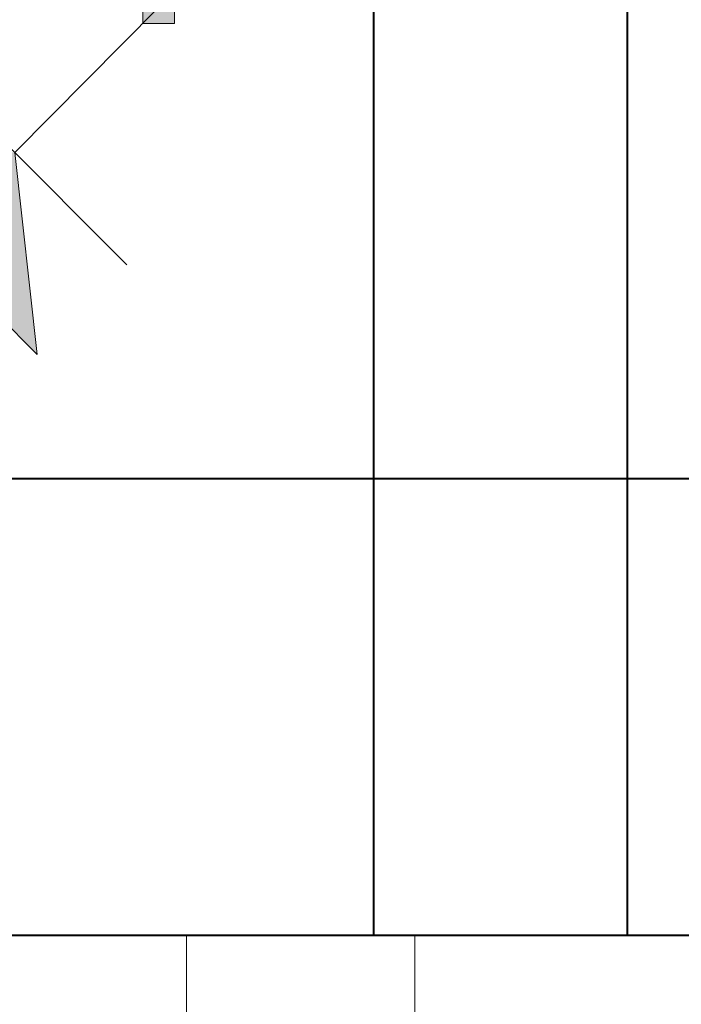
# Model space of a CAD drawing. Units: inches. Extents: x 459864 to 460310, y 324185 to 324787.
# Tile 66 of 112: x 460114.14 to 460127.18, y 324282.12 to 324301.53. Entities that reach past the tile are written whole.
import ezdxf

# ---------------------------------------------------------------- set-up
doc = ezdxf.new("R2010")
doc.units = ezdxf.units.IN
for name, color, linetype, lineweight in [('A-ANNO-DIMS', 2, 'Continuous', 18), ('A-FURN', 8, 'Continuous', 18), ('A-WALL', 7, 'Continuous', 40), ('L-HRDS', 9, 'Continuous', 18), ('L-SITE-PATT', 252, 'Continuous', 13)]:
    doc.layers.add(name, color=color, linetype=linetype, lineweight=lineweight)
doc.styles.get("Standard").update_dxf_attribs({"font": 'arial.ttf'})
doc.dimstyles.new('ISO-25', dxfattribs={"dimtxt": 6, "dimasz": 2.5, "dimexe": 1.25, "dimexo": 0.625, "dimtad": 1, "dimdec": 1, "dimlunit": 3, "dimtxsty": 'Standard', "dimcen": 2.5, "dimadec": 0, "dimazin": 0, "dimtfac": 1, "dimtdec": 1, "dimtmove": 0, "dimatfit": 3, "dimfxl": 1, "dimarcsym": 0})

# ---------------------------------------------------------------- blocks, each defined once
blk = doc.blocks.new('Full Wave Bridge')
for p, q in [((0.486497, -0.114373), (0.6, 0)), ((0.574885, -0.202762), (0.398108, -0.025985)), ((0.504174, -0.273472), (0.327398, -0.096695)), ((0.486497, -0.114373), (0.504174, -0.273472))]:
    blk.add_line(p, q)
blk.add_lwpolyline([(0.5875, -0.0125), (0.5875, 0.0125), (0.6125, 0.0125), (0.6125, -0.0125)], close=True)
for points in [[(0.6125, -0.0125), (0.6125, 0.0125), (0.5875, 0.0125)], [(0.5875, 0.0125), (0.5875, -0.0125), (0.6125, -0.0125)], [(0.327398, -0.096695), (0.486497, -0.114373), (0.504174, -0.273472)]]:
    blk.add_solid(points)
blk = doc.blocks.new('*D28')
at = {"layer": 'A-ANNO-DIMS', "color": 0, "lineweight": -2, "transparency": 16777216}
for p, q in [((460148.65, 324370.7), (460136.025, 324370.7)), ((460137.275, 324368.2), (460137.275, 324293.2)), ((460148.65, 324290.7), (460136.025, 324290.7)), ((460137.275, 324290.7), (460137.275, 324198.69))]:
    blk.add_line(p, q, dxfattribs=at)
at = {"layer": 'A-ANNO-DIMS', "color": 0, "transparency": 16777216}
for points in [[(460136.858, 324368.2), (460137.692, 324368.2), (460137.275, 324370.7)], [(460136.858, 324293.2), (460137.692, 324293.2), (460137.275, 324290.7)]]:
    blk.add_solid(points, dxfattribs=at)
at = {"layer": 'Defpoints', "color": 0, "transparency": 16777216}
for p in [(460149.275, 324370.7), (460137.275, 324290.7), (460149.275, 324290.7)]:
    blk.add_point(p, dxfattribs=at)
at = {"layer": 'A-ANNO-DIMS', "color": 0, "transparency": 16777216, "insert": (460133.363, 324243.445), "char_height": 6, "attachment_point": 5, "rotation": 90}
blk.add_mtext('QUEEN BED 6\'-8" TYP.', dxfattribs=at)

msp = doc.modelspace()

# ---------------------------------------------------------------- hatches: boundary and pattern name
at = {"layer": 'L-SITE-PATT'}
h = msp.add_hatch(dxfattribs=at)
h.set_pattern_fill('DOTS', color=256)
h.paths.add_polyline_path([(460269.804, 324283.483), (460247.115, 324283.483), (460121.929, 324283.483), (460121.929, 324252.473), (460117.429, 324252.473), (460110.124, 324252.473), (460110.124, 324243.287), (460080.83, 324243.287), (460080.83, 324252.473), (460061.115, 324252.473), (460061.115, 324251.882), (460077.909, 324251.882), (460077.909, 324199.483), (460080.83, 324199.483), (460080.83, 324207.553), (460110.124, 324207.553), (460110.124, 324199.483), (460110.813, 324199.483), (460262.115, 324199.483), (460269.804, 324199.483)], flags=17)
edge = h.paths.add_edge_path(flags=0)
edge.add_ellipse((460222.59, 324263.813), major_axis=(-8.485, 8.485), ratio=1, start_angle=405, end_angle=495, ccw=False)
edge.add_line((460214.821, 324254.66), (460214.832, 324254.666))
edge.add_ellipse((460222.59, 324263.813), major_axis=(-8.485, 8.485), ratio=1, start_angle=405, end_angle=495, ccw=False)
edge.add_line((460210.759, 324261.781), (460210.768, 324261.787))
edge.add_ellipse((460222.59, 324263.813), major_axis=(-8.485, 8.485), ratio=1, start_angle=405, end_angle=495, ccw=False)
edge.add_ellipse((460222.59, 324263.813), major_axis=(-8.485, 8.485), ratio=1, start_angle=392.754, end_angle=405, ccw=False)
edge.add_ellipse((460222.59, 324263.813), major_axis=(-8.485, 8.485), ratio=1, start_angle=380.9347, end_angle=392.754, ccw=False)
edge.add_line((460211.337, 324267.985), (460211.34, 324267.985))
edge.add_ellipse((460222.59, 324263.813), major_axis=(-8.485, 8.485), ratio=1, start_angle=380.9347, end_angle=392.754, ccw=False)
edge.add_ellipse((460222.59, 324263.813), major_axis=(-8.485, 8.485), ratio=1, start_angle=347.9015, end_angle=380.9347, ccw=False)
edge.add_ellipse((460222.59, 324263.813), major_axis=(-8.485, 8.485), ratio=1, start_angle=327.0619, end_angle=347.9015, ccw=False)
edge.add_ellipse((460222.59, 324263.813), major_axis=(-8.485, 8.485), ratio=1, start_angle=278.3246, end_angle=327.0619, ccw=False)
edge.add_line((460225.158, 324275.536), (460225.158, 324275.535))
edge.add_ellipse((460222.59, 324263.813), major_axis=(-8.485, 8.485), ratio=1, start_angle=278.3246, end_angle=327.0619, ccw=False)
edge.add_ellipse((460222.59, 324263.813), major_axis=(-8.485, 8.485), ratio=1, start_angle=260.6436, end_angle=278.3246, ccw=False)
edge.add_ellipse((460222.59, 324263.813), major_axis=(-8.485, 8.485), ratio=1, start_angle=225, end_angle=260.6436, ccw=False)
edge.add_line((460234.509, 324265.243), (460234.501, 324265.239))
edge.add_ellipse((460222.59, 324263.813), major_axis=(-8.485, 8.485), ratio=1, start_angle=225, end_angle=260.6436, ccw=False)
edge.add_ellipse((460222.59, 324263.813), major_axis=(-8.485, 8.485), ratio=1, start_angle=495, end_angle=585, ccw=False)
edge.add_line((460234.437, 324261.861), (460234.424, 324261.858))
edge.add_ellipse((460222.59, 324263.813), major_axis=(-8.485, 8.485), ratio=1, start_angle=495, end_angle=585, ccw=False)
edge.add_line((460227.95, 324253.067), (460227.946, 324253.083))
edge.add_ellipse((460222.59, 324263.813), major_axis=(-8.485, 8.485), ratio=1, start_angle=495, end_angle=585, ccw=False)
edge.add_line((460226.223, 324252.369), (460226.211, 324252.38))
edge.add_ellipse((460222.59, 324263.813), major_axis=(-8.485, 8.485), ratio=1, start_angle=495, end_angle=585, ccw=False)
h.paths.add_polyline_path([(460219.651, 324254.347), (460218.461, 324253.545), (460218.275, 324254.789), (460219.642, 324256.542), (460219.625, 324260.848), (460216.11, 324257.333), (460214.35, 324256.978), (460215.416, 324259.356), (460212.524, 324258.496), (460213.137, 324259.93), (460218.507, 324263.813), (460222.59, 324263.813), (460222.59, 324267.807), (460218.176, 324272.212), (460219.026, 324274.639), (460222.59, 324272.811), (460222.59, 324275.423), (460223.057, 324274.825), (460222.675, 324273.492), (460225.912, 324267.135), (460219.625, 324260.848)], flags=0)
edge = h.paths.add_edge_path(flags=0)
edge.add_ellipse((460194.576, 324264.046), major_axis=(-8.485, 8.485), ratio=1, start_angle=495, end_angle=585, ccw=False)
edge.add_line((460199.936, 324253.3), (460199.932, 324253.316))
edge.add_ellipse((460194.576, 324264.046), major_axis=(-8.485, 8.485), ratio=1, start_angle=495, end_angle=585, ccw=False)
edge.add_line((460198.208, 324252.603), (460198.196, 324252.613))
edge.add_ellipse((460194.576, 324264.046), major_axis=(-8.485, 8.485), ratio=1, start_angle=495, end_angle=585, ccw=False)
edge.add_ellipse((460194.576, 324264.046), major_axis=(-8.485, 8.485), ratio=1, start_angle=405, end_angle=495, ccw=False)
edge.add_line((460186.806, 324254.893), (460186.817, 324254.899))
edge.add_ellipse((460194.576, 324264.046), major_axis=(-8.485, 8.485), ratio=1, start_angle=405, end_angle=495, ccw=False)
edge.add_line((460182.744, 324262.014), (460182.753, 324262.02))
edge.add_ellipse((460194.576, 324264.046), major_axis=(-8.485, 8.485), ratio=1, start_angle=405, end_angle=495, ccw=False)
edge.add_ellipse((460194.576, 324264.046), major_axis=(-8.485, 8.485), ratio=1, start_angle=392.754, end_angle=405, ccw=False)
edge.add_ellipse((460194.576, 324264.046), major_axis=(-8.485, 8.485), ratio=1, start_angle=380.9347, end_angle=392.754, ccw=False)
edge.add_line((460183.323, 324268.218), (460183.326, 324268.218))
edge.add_ellipse((460194.576, 324264.046), major_axis=(-8.485, 8.485), ratio=1, start_angle=380.9347, end_angle=392.754, ccw=False)
edge.add_ellipse((460194.576, 324264.046), major_axis=(-8.485, 8.485), ratio=1, start_angle=347.9015, end_angle=380.9347, ccw=False)
edge.add_ellipse((460194.576, 324264.046), major_axis=(-8.485, 8.485), ratio=1, start_angle=327.0619, end_angle=347.9015, ccw=False)
edge.add_ellipse((460194.576, 324264.046), major_axis=(-8.485, 8.485), ratio=1, start_angle=278.3246, end_angle=327.0619, ccw=False)
edge.add_line((460197.144, 324275.769), (460197.143, 324275.768))
edge.add_ellipse((460194.576, 324264.046), major_axis=(-8.485, 8.485), ratio=1, start_angle=278.3246, end_angle=327.0619, ccw=False)
edge.add_ellipse((460194.576, 324264.046), major_axis=(-8.485, 8.485), ratio=1, start_angle=260.6436, end_angle=278.3246, ccw=False)
edge.add_ellipse((460194.576, 324264.046), major_axis=(-8.485, 8.485), ratio=1, start_angle=225, end_angle=260.6436, ccw=False)
edge.add_line((460206.494, 324265.476), (460206.487, 324265.473))
edge.add_ellipse((460194.576, 324264.046), major_axis=(-8.485, 8.485), ratio=1, start_angle=225, end_angle=260.6436, ccw=False)
edge.add_ellipse((460194.576, 324264.046), major_axis=(-8.485, 8.485), ratio=1, start_angle=495, end_angle=585, ccw=False)
edge.add_line((460206.422, 324262.094), (460206.409, 324262.091))
h.paths.add_polyline_path([(460191.61, 324261.081), (460191.637, 324254.58), (460190.447, 324253.778), (460190.261, 324255.023), (460191.628, 324256.775), (460191.61, 324261.081), (460188.096, 324257.566), (460186.335, 324257.211), (460187.402, 324259.589), (460184.509, 324258.729), (460185.123, 324260.163), (460190.493, 324264.046), (460194.576, 324264.046), (460194.576, 324268.04), (460190.161, 324272.446), (460191.011, 324274.872), (460194.576, 324273.044), (460194.576, 324275.657), (460195.043, 324275.058), (460194.661, 324273.725), (460197.897, 324267.368)], flags=0)
edge = h.paths.add_edge_path(flags=0)
edge.add_ellipse((460252.912, 324263.578), major_axis=(-8.485, 8.485), ratio=1, start_angle=405, end_angle=495, ccw=False)
edge.add_line((460241.081, 324261.545), (460241.089, 324261.551))
edge.add_ellipse((460252.912, 324263.578), major_axis=(-8.485, 8.485), ratio=1, start_angle=405, end_angle=495, ccw=False)
edge.add_ellipse((460252.912, 324263.578), major_axis=(-8.485, 8.485), ratio=1, start_angle=392.754, end_angle=405, ccw=False)
edge.add_ellipse((460252.912, 324263.578), major_axis=(-8.485, 8.485), ratio=1, start_angle=380.9347, end_angle=392.754, ccw=False)
edge.add_line((460241.659, 324267.749), (460241.662, 324267.749))
edge.add_ellipse((460252.912, 324263.578), major_axis=(-8.485, 8.485), ratio=1, start_angle=380.9347, end_angle=392.754, ccw=False)
edge.add_ellipse((460252.912, 324263.578), major_axis=(-8.485, 8.485), ratio=1, start_angle=347.9015, end_angle=380.9347, ccw=False)
edge.add_ellipse((460252.912, 324263.578), major_axis=(-8.485, 8.485), ratio=1, start_angle=327.0619, end_angle=347.9015, ccw=False)
edge.add_ellipse((460252.912, 324263.578), major_axis=(-8.485, 8.485), ratio=1, start_angle=278.3246, end_angle=327.0619, ccw=False)
edge.add_line((460255.48, 324275.3), (460255.479, 324275.299))
edge.add_ellipse((460252.912, 324263.578), major_axis=(-8.485, 8.485), ratio=1, start_angle=278.3246, end_angle=327.0619, ccw=False)
edge.add_ellipse((460252.912, 324263.578), major_axis=(-8.485, 8.485), ratio=1, start_angle=260.6436, end_angle=278.3246, ccw=False)
edge.add_ellipse((460252.912, 324263.578), major_axis=(-8.485, 8.485), ratio=1, start_angle=225, end_angle=260.6436, ccw=False)
edge.add_line((460264.83, 324265.007), (460264.823, 324265.004))
edge.add_ellipse((460252.912, 324263.578), major_axis=(-8.485, 8.485), ratio=1, start_angle=225, end_angle=260.6436, ccw=False)
edge.add_ellipse((460252.912, 324263.578), major_axis=(-8.485, 8.485), ratio=1, start_angle=495, end_angle=585, ccw=False)
edge.add_line((460264.758, 324261.626), (460264.745, 324261.622))
edge.add_ellipse((460252.912, 324263.578), major_axis=(-8.485, 8.485), ratio=1, start_angle=495, end_angle=585, ccw=False)
edge.add_line((460258.272, 324252.832), (460258.268, 324252.848))
edge.add_ellipse((460252.912, 324263.578), major_axis=(-8.485, 8.485), ratio=1, start_angle=495, end_angle=585, ccw=False)
edge.add_line((460256.545, 324252.134), (460256.533, 324252.144))
edge.add_ellipse((460252.912, 324263.578), major_axis=(-8.485, 8.485), ratio=1, start_angle=495, end_angle=585, ccw=False)
edge.add_ellipse((460252.912, 324263.578), major_axis=(-8.485, 8.485), ratio=1, start_angle=405, end_angle=495, ccw=False)
edge.add_line((460245.143, 324254.424), (460245.153, 324254.43))
h.paths.add_polyline_path([(460244.672, 324256.742), (460245.738, 324259.12), (460242.846, 324258.26), (460243.459, 324259.694), (460248.829, 324263.578), (460252.912, 324263.578), (460252.912, 324267.571), (460248.497, 324271.977), (460249.348, 324274.403), (460252.912, 324272.576), (460252.912, 324275.188), (460253.379, 324274.589), (460252.997, 324273.257), (460256.233, 324266.899), (460249.946, 324260.612), (460249.973, 324254.111), (460248.783, 324253.309), (460248.597, 324254.554), (460249.964, 324256.306), (460249.946, 324260.612), (460246.432, 324257.097)], flags=0)
edge = h.paths.add_edge_path(flags=0)
edge.add_ellipse((460167.439, 324262.833), major_axis=(-8.485, 8.485), ratio=1, start_angle=495, end_angle=585, ccw=False)
edge.add_line((460172.799, 324252.087), (460172.795, 324252.103))
edge.add_ellipse((460167.439, 324262.833), major_axis=(-8.485, 8.485), ratio=1, start_angle=495, end_angle=585, ccw=False)
edge.add_line((460171.071, 324251.389), (460171.059, 324251.399))
edge.add_ellipse((460167.439, 324262.833), major_axis=(-8.485, 8.485), ratio=1, start_angle=495, end_angle=585, ccw=False)
edge.add_ellipse((460167.439, 324262.833), major_axis=(-8.485, 8.485), ratio=1, start_angle=405, end_angle=495, ccw=False)
edge.add_line((460159.669, 324253.679), (460159.68, 324253.685))
edge.add_ellipse((460167.439, 324262.833), major_axis=(-8.485, 8.485), ratio=1, start_angle=405, end_angle=495, ccw=False)
edge.add_line((460155.607, 324260.8), (460155.616, 324260.806))
edge.add_ellipse((460167.439, 324262.833), major_axis=(-8.485, 8.485), ratio=1, start_angle=405, end_angle=495, ccw=False)
edge.add_ellipse((460167.439, 324262.833), major_axis=(-8.485, 8.485), ratio=1, start_angle=392.754, end_angle=405, ccw=False)
edge.add_ellipse((460167.439, 324262.833), major_axis=(-8.485, 8.485), ratio=1, start_angle=380.9347, end_angle=392.754, ccw=False)
edge.add_line((460156.185, 324267.005), (460156.189, 324267.005))
edge.add_ellipse((460167.439, 324262.833), major_axis=(-8.485, 8.485), ratio=1, start_angle=380.9347, end_angle=392.754, ccw=False)
edge.add_ellipse((460167.439, 324262.833), major_axis=(-8.485, 8.485), ratio=1, start_angle=347.9015, end_angle=380.9347, ccw=False)
edge.add_ellipse((460167.439, 324262.833), major_axis=(-8.485, 8.485), ratio=1, start_angle=327.0619, end_angle=347.9015, ccw=False)
edge.add_ellipse((460167.439, 324262.833), major_axis=(-8.485, 8.485), ratio=1, start_angle=278.3246, end_angle=327.0619, ccw=False)
edge.add_line((460170.007, 324274.556), (460170.006, 324274.554))
edge.add_ellipse((460167.439, 324262.833), major_axis=(-8.485, 8.485), ratio=1, start_angle=278.3246, end_angle=327.0619, ccw=False)
edge.add_ellipse((460167.439, 324262.833), major_axis=(-8.485, 8.485), ratio=1, start_angle=260.6436, end_angle=278.3246, ccw=False)
edge.add_ellipse((460167.439, 324262.833), major_axis=(-8.485, 8.485), ratio=1, start_angle=225, end_angle=260.6436, ccw=False)
edge.add_line((460179.357, 324264.262), (460179.35, 324264.259))
edge.add_ellipse((460167.439, 324262.833), major_axis=(-8.485, 8.485), ratio=1, start_angle=225, end_angle=260.6436, ccw=False)
edge.add_ellipse((460167.439, 324262.833), major_axis=(-8.485, 8.485), ratio=1, start_angle=495, end_angle=585, ccw=False)
edge.add_line((460179.285, 324260.881), (460179.272, 324260.877))
h.paths.add_polyline_path([(460164.473, 324259.867), (460164.5, 324253.366), (460163.31, 324252.565), (460163.124, 324253.809), (460164.491, 324255.561), (460164.473, 324259.867), (460160.958, 324256.353), (460159.198, 324255.998), (460160.265, 324258.375), (460157.372, 324257.515), (460157.986, 324258.949), (460163.356, 324262.833), (460167.439, 324262.833), (460167.439, 324266.826), (460163.024, 324271.232), (460163.874, 324273.659), (460167.439, 324271.831), (460167.439, 324274.443), (460167.905, 324273.844), (460167.524, 324272.512), (460170.76, 324266.154)], flags=0)
edge = h.paths.add_edge_path(flags=0)
edge.add_ellipse((460140.758, 324262.37), major_axis=(-8.485, 8.485), ratio=1, start_angle=495, end_angle=585, ccw=False)
edge.add_line((460146.118, 324251.624), (460146.114, 324251.639))
edge.add_ellipse((460140.758, 324262.37), major_axis=(-8.485, 8.485), ratio=1, start_angle=495, end_angle=585, ccw=False)
edge.add_line((460144.391, 324250.926), (460144.379, 324250.936))
edge.add_ellipse((460140.758, 324262.37), major_axis=(-8.485, 8.485), ratio=1, start_angle=495, end_angle=585, ccw=False)
edge.add_ellipse((460140.758, 324262.37), major_axis=(-8.485, 8.485), ratio=1, start_angle=405, end_angle=495, ccw=False)
edge.add_line((460132.989, 324253.216), (460132.999, 324253.222))
edge.add_ellipse((460140.758, 324262.37), major_axis=(-8.485, 8.485), ratio=1, start_angle=405, end_angle=495, ccw=False)
edge.add_line((460128.927, 324260.337), (460128.935, 324260.343))
edge.add_ellipse((460140.758, 324262.37), major_axis=(-8.485, 8.485), ratio=1, start_angle=405, end_angle=495, ccw=False)
edge.add_ellipse((460140.758, 324262.37), major_axis=(-8.485, 8.485), ratio=1, start_angle=392.754, end_angle=405, ccw=False)
edge.add_ellipse((460140.758, 324262.37), major_axis=(-8.485, 8.485), ratio=1, start_angle=380.9347, end_angle=392.754, ccw=False)
edge.add_line((460129.505, 324266.541), (460129.508, 324266.541))
edge.add_ellipse((460140.758, 324262.37), major_axis=(-8.485, 8.485), ratio=1, start_angle=380.9347, end_angle=392.754, ccw=False)
edge.add_ellipse((460140.758, 324262.37), major_axis=(-8.485, 8.485), ratio=1, start_angle=347.9015, end_angle=380.9347, ccw=False)
edge.add_ellipse((460140.758, 324262.37), major_axis=(-8.485, 8.485), ratio=1, start_angle=327.0619, end_angle=347.9015, ccw=False)
edge.add_ellipse((460140.758, 324262.37), major_axis=(-8.485, 8.485), ratio=1, start_angle=278.3246, end_angle=327.0619, ccw=False)
edge.add_line((460143.326, 324274.092), (460143.325, 324274.091))
edge.add_ellipse((460140.758, 324262.37), major_axis=(-8.485, 8.485), ratio=1, start_angle=278.3246, end_angle=327.0619, ccw=False)
edge.add_ellipse((460140.758, 324262.37), major_axis=(-8.485, 8.485), ratio=1, start_angle=260.6436, end_angle=278.3246, ccw=False)
edge.add_ellipse((460140.758, 324262.37), major_axis=(-8.485, 8.485), ratio=1, start_angle=225, end_angle=260.6436, ccw=False)
edge.add_line((460152.677, 324263.799), (460152.669, 324263.796))
edge.add_ellipse((460140.758, 324262.37), major_axis=(-8.485, 8.485), ratio=1, start_angle=225, end_angle=260.6436, ccw=False)
edge.add_ellipse((460140.758, 324262.37), major_axis=(-8.485, 8.485), ratio=1, start_angle=495, end_angle=585, ccw=False)
edge.add_line((460152.604, 324260.418), (460152.592, 324260.414))
h.paths.add_polyline_path([(460137.792, 324259.404), (460137.819, 324252.903), (460136.629, 324252.101), (460136.443, 324253.346), (460137.81, 324255.098), (460137.792, 324259.404), (460134.278, 324255.889), (460132.518, 324255.534), (460133.584, 324257.912), (460130.692, 324257.052), (460131.305, 324258.486), (460136.675, 324262.37), (460140.758, 324262.37), (460140.758, 324266.363), (460136.343, 324270.769), (460137.194, 324273.195), (460140.758, 324271.367), (460140.758, 324273.98), (460141.225, 324273.381), (460140.843, 324272.049), (460144.079, 324265.691)], flags=0)
h.paths.add_polyline_path([(460110.124, 324227.414), (460080.83, 324227.414), (460080.83, 324235.484), (460110.124, 324235.484)], flags=16)
h.paths.add_polyline_path([(460110.124, 324220.797), (460110.124, 324212.727), (460080.83, 324212.727), (460080.83, 324220.797)], flags=16)
h.paths.add_polyline_path([(460269.804, 324283.483), (460247.115, 324283.483), (460121.929, 324283.483), (460121.929, 324252.473), (460117.429, 324252.473), (460110.124, 324252.473), (460110.124, 324243.287), (460080.83, 324243.287), (460080.83, 324252.473), (460061.115, 324252.473), (460061.115, 324251.882), (460077.909, 324251.882), (460077.909, 324199.483), (460080.83, 324199.483), (460080.83, 324207.553), (460110.124, 324207.553), (460110.124, 324199.483), (460262.115, 324199.483), (460269.804, 324199.483)], flags=17)
h.paths.add_polyline_path([(460219.651, 324254.347), (460218.461, 324253.545), (460218.275, 324254.789), (460219.642, 324256.542), (460219.625, 324260.848), (460216.11, 324257.333), (460214.35, 324256.978), (460215.416, 324259.356), (460212.524, 324258.496), (460213.137, 324259.93), (460218.507, 324263.813), (460222.59, 324263.813), (460220.18, 324266.223), (460215.461, 324265.308), (460211.835, 324266.137), (460216.247, 324267.985), (460218.418, 324267.985), (460222.59, 324263.813), (460222.59, 324267.807), (460218.176, 324272.212), (460219.026, 324274.639), (460222.59, 324272.811), (460222.59, 324275.423), (460223.057, 324274.825), (460222.675, 324273.492), (460225.912, 324267.135), (460222.59, 324263.813), (460231.383, 324263.813), (460228.485, 324262.488), (460224.425, 324261.978), (460228.68, 324257.724), (460228.966, 324254.791), (460227.142, 324256.537), (460227.542, 324254.819), (460227.333, 324253.614), (460222.59, 324259.985), (460222.59, 324255.497), (460221.377, 324256.541), (460220.576, 324261.799), (460219.625, 324260.848)], flags=0)
h.paths.add_polyline_path([(460199.127, 324256.77), (460199.528, 324255.052), (460199.319, 324253.848), (460194.576, 324260.218), (460194.576, 324255.73), (460193.363, 324256.774), (460192.561, 324262.032), (460191.61, 324261.081), (460191.637, 324254.58), (460190.447, 324253.778), (460190.261, 324255.023), (460191.628, 324256.775), (460191.61, 324261.081), (460188.096, 324257.566), (460186.335, 324257.211), (460187.402, 324259.589), (460184.509, 324258.729), (460185.123, 324260.163), (460190.493, 324264.046), (460194.576, 324264.046), (460192.166, 324266.456), (460187.446, 324265.541), (460183.82, 324266.37), (460188.232, 324268.218), (460190.404, 324268.218), (460194.576, 324264.046), (460194.576, 324268.04), (460190.161, 324272.446), (460191.011, 324274.872), (460194.576, 324273.044), (460194.576, 324275.657), (460195.043, 324275.058), (460194.661, 324273.725), (460197.897, 324267.368), (460194.576, 324264.046), (460203.368, 324264.046), (460200.47, 324262.721), (460196.411, 324262.212), (460200.665, 324257.957), (460200.951, 324255.024)], flags=0)
h.paths.add_polyline_path([(460244.672, 324256.742), (460245.738, 324259.12), (460242.846, 324258.26), (460243.459, 324259.694), (460248.829, 324263.578), (460252.912, 324263.578), (460250.502, 324265.987), (460245.783, 324265.072), (460242.156, 324265.901), (460246.568, 324267.749), (460248.74, 324267.749), (460252.912, 324263.578), (460252.912, 324267.571), (460248.497, 324271.977), (460249.348, 324274.403), (460252.912, 324272.576), (460252.912, 324275.188), (460253.379, 324274.589), (460252.997, 324273.257), (460256.233, 324266.899), (460252.912, 324263.578), (460261.705, 324263.578), (460258.806, 324262.252), (460254.747, 324261.743), (460259.002, 324257.488), (460259.288, 324254.555), (460257.463, 324256.301), (460257.864, 324254.583), (460257.655, 324253.379), (460252.912, 324259.749), (460252.912, 324255.261), (460251.699, 324256.305), (460250.897, 324261.563), (460249.946, 324260.612), (460249.973, 324254.111), (460248.783, 324253.309), (460248.597, 324254.554), (460249.964, 324256.306), (460249.946, 324260.612), (460246.432, 324257.097)], flags=0)
h.paths.add_polyline_path([(460173.528, 324256.743), (460173.814, 324253.811), (460171.99, 324255.556), (460172.39, 324253.838), (460172.182, 324252.634), (460167.439, 324259.004), (460167.439, 324254.516), (460166.226, 324255.56), (460165.424, 324260.818), (460164.473, 324259.867), (460164.5, 324253.366), (460163.31, 324252.565), (460163.124, 324253.809), (460164.491, 324255.561), (460164.473, 324259.867), (460160.958, 324256.353), (460159.198, 324255.998), (460160.265, 324258.375), (460157.372, 324257.515), (460157.986, 324258.949), (460163.356, 324262.833), (460167.439, 324262.833), (460165.029, 324265.243), (460160.309, 324264.327), (460156.683, 324265.156), (460161.095, 324267.005), (460163.267, 324267.005), (460167.439, 324262.833), (460167.439, 324266.826), (460163.024, 324271.232), (460163.874, 324273.659), (460167.439, 324271.831), (460167.439, 324274.443), (460167.905, 324273.844), (460167.524, 324272.512), (460170.76, 324266.154), (460167.439, 324262.833), (460176.231, 324262.833), (460173.333, 324261.507), (460169.274, 324260.998)], flags=0)
h.paths.add_polyline_path([(460146.848, 324256.28), (460147.134, 324253.347), (460145.31, 324255.093), (460145.71, 324253.375), (460145.501, 324252.171), (460140.758, 324258.541), (460140.758, 324254.053), (460139.545, 324255.097), (460138.744, 324260.355), (460137.792, 324259.404), (460137.819, 324252.903), (460136.629, 324252.101), (460136.443, 324253.346), (460137.81, 324255.098), (460137.792, 324259.404), (460134.278, 324255.889), (460132.518, 324255.534), (460133.584, 324257.912), (460130.692, 324257.052), (460131.305, 324258.486), (460136.675, 324262.37), (460140.758, 324262.37), (460138.348, 324264.779), (460133.629, 324263.864), (460130.002, 324264.693), (460134.414, 324266.541), (460136.586, 324266.541), (460140.758, 324262.37), (460140.758, 324266.363), (460136.343, 324270.769), (460137.194, 324273.195), (460140.758, 324271.367), (460140.758, 324273.98), (460141.225, 324273.381), (460140.843, 324272.049), (460144.079, 324265.691), (460140.758, 324262.37), (460149.551, 324262.37), (460146.653, 324261.044), (460142.593, 324260.535)], flags=0)
edge = h.paths.add_edge_path()
edge.add_line((460269.804, 324272.549), (460260.881, 324272.549))
edge.add_ellipse((460252.912, 324263.578), major_axis=(-8.485, 8.485), ratio=1, start_angle=260.6436, end_angle=273.3846, ccw=False)
edge.add_line((460262.283, 324271.092), (460262.261, 324271.091))
edge.add_ellipse((460252.912, 324263.578), major_axis=(-8.485, 8.485), ratio=1, start_angle=260.6436, end_angle=273.3846, ccw=False)
edge.add_ellipse((460252.912, 324263.578), major_axis=(-8.485, 8.485), ratio=1, start_angle=225, end_angle=260.6436, ccw=False)
edge.add_line((460263.609, 324269.063), (460263.572, 324269.058))
edge.add_ellipse((460252.912, 324263.578), major_axis=(-8.485, 8.485), ratio=1, start_angle=225, end_angle=260.6436, ccw=False)
edge.add_line((460264.615, 324266.306), (460264.585, 324266.305))
edge.add_ellipse((460252.912, 324263.578), major_axis=(-8.485, 8.485), ratio=1, start_angle=225, end_angle=260.6436, ccw=False)
edge.add_line((460264.83, 324265.007), (460264.823, 324265.004))
edge.add_ellipse((460252.912, 324263.578), major_axis=(-8.485, 8.485), ratio=1, start_angle=225, end_angle=260.6436, ccw=False)
edge.add_ellipse((460252.912, 324263.578), major_axis=(-8.485, 8.485), ratio=1, start_angle=495, end_angle=585, ccw=False)
edge.add_line((460264.758, 324261.626), (460264.745, 324261.622))
edge.add_ellipse((460252.912, 324263.578), major_axis=(-8.485, 8.485), ratio=1, start_angle=495, end_angle=585, ccw=False)
edge.add_line((460263.442, 324257.739), (460263.389, 324257.779))
edge.add_ellipse((460252.912, 324263.578), major_axis=(-8.485, 8.485), ratio=1, start_angle=495, end_angle=585, ccw=False)
edge.add_line((460258.128, 324252.744), (460258.102, 324252.779))
edge.add_ellipse((460252.912, 324263.578), major_axis=(-8.485, 8.485), ratio=1, start_angle=495, end_angle=585, ccw=False)
edge.add_line((460256.545, 324252.134), (460256.533, 324252.144))
edge.add_ellipse((460252.912, 324263.578), major_axis=(-8.485, 8.485), ratio=1, start_angle=495, end_angle=585, ccw=False)
edge.add_ellipse((460252.912, 324263.578), major_axis=(-8.485, 8.485), ratio=1, start_angle=405, end_angle=495, ccw=False)
edge.add_line((460250.594, 324251.78), (460250.605, 324251.82))
edge.add_ellipse((460252.912, 324263.578), major_axis=(-8.485, 8.485), ratio=1, start_angle=405, end_angle=495, ccw=False)
edge.add_line((460245.143, 324254.424), (460245.153, 324254.43))
edge.add_ellipse((460252.912, 324263.578), major_axis=(-8.485, 8.485), ratio=1, start_angle=405, end_angle=495, ccw=False)
edge.add_line((460243.525, 324256.059), (460243.56, 324256.091))
edge.add_ellipse((460252.912, 324263.578), major_axis=(-8.485, 8.485), ratio=1, start_angle=405, end_angle=495, ccw=False)
edge.add_line((460241.44, 324259.893), (460241.522, 324259.896))
edge.add_ellipse((460252.912, 324263.578), major_axis=(-8.485, 8.485), ratio=1, start_angle=405, end_angle=495, ccw=False)
edge.add_line((460241.081, 324261.545), (460241.089, 324261.551))
edge.add_ellipse((460252.912, 324263.578), major_axis=(-8.485, 8.485), ratio=1, start_angle=405, end_angle=495, ccw=False)
edge.add_ellipse((460252.912, 324263.578), major_axis=(-8.485, 8.485), ratio=1, start_angle=392.754, end_angle=405, ccw=False)
edge.add_line((460241.05, 324265.438), (460241.063, 324265.443))
edge.add_ellipse((460252.912, 324263.578), major_axis=(-8.485, 8.485), ratio=1, start_angle=392.754, end_angle=405, ccw=False)
edge.add_ellipse((460252.912, 324263.578), major_axis=(-8.485, 8.485), ratio=1, start_angle=380.9347, end_angle=392.754, ccw=False)
edge.add_line((460241.452, 324267.176), (460241.469, 324267.171))
edge.add_ellipse((460252.912, 324263.578), major_axis=(-8.485, 8.485), ratio=1, start_angle=380.9347, end_angle=392.754, ccw=False)
edge.add_line((460241.659, 324267.749), (460241.662, 324267.749))
edge.add_ellipse((460252.912, 324263.578), major_axis=(-8.485, 8.485), ratio=1, start_angle=380.9347, end_angle=392.754, ccw=False)
edge.add_ellipse((460252.912, 324263.578), major_axis=(-8.485, 8.485), ratio=1, start_angle=356.6154, end_angle=380.9347, ccw=False)
edge.add_line((460244.88, 324272.488), (460244.713, 324272.549))
edge.add_line((460244.713, 324272.549), (460230.817, 324272.549))
edge.add_ellipse((460222.59, 324263.813), major_axis=(-8.485, 8.485), ratio=1, start_angle=260.6436, end_angle=271.7178, ccw=False)
edge.add_ellipse((460222.59, 324263.813), major_axis=(-8.485, 8.485), ratio=1, start_angle=225, end_angle=260.6436, ccw=False)
edge.add_line((460233.287, 324269.299), (460233.25, 324269.294))
edge.add_ellipse((460222.59, 324263.813), major_axis=(-8.485, 8.485), ratio=1, start_angle=225, end_angle=260.6436, ccw=False)
edge.add_line((460234.294, 324266.541), (460234.264, 324266.541))
edge.add_ellipse((460222.59, 324263.813), major_axis=(-8.485, 8.485), ratio=1, start_angle=225, end_angle=260.6436, ccw=False)
edge.add_line((460234.509, 324265.243), (460234.501, 324265.239))
edge.add_ellipse((460222.59, 324263.813), major_axis=(-8.485, 8.485), ratio=1, start_angle=225, end_angle=260.6436, ccw=False)
edge.add_ellipse((460222.59, 324263.813), major_axis=(-8.485, 8.485), ratio=1, start_angle=495, end_angle=585, ccw=False)
edge.add_line((460234.437, 324261.861), (460234.424, 324261.858))
edge.add_ellipse((460222.59, 324263.813), major_axis=(-8.485, 8.485), ratio=1, start_angle=495, end_angle=585, ccw=False)
edge.add_line((460233.121, 324257.975), (460233.068, 324258.015))
edge.add_ellipse((460222.59, 324263.813), major_axis=(-8.485, 8.485), ratio=1, start_angle=495, end_angle=585, ccw=False)
edge.add_line((460227.806, 324252.979), (460227.78, 324253.014))
edge.add_ellipse((460222.59, 324263.813), major_axis=(-8.485, 8.485), ratio=1, start_angle=495, end_angle=585, ccw=False)
edge.add_line((460226.223, 324252.369), (460226.211, 324252.38))
edge.add_ellipse((460222.59, 324263.813), major_axis=(-8.485, 8.485), ratio=1, start_angle=495, end_angle=585, ccw=False)
edge.add_ellipse((460222.59, 324263.813), major_axis=(-8.485, 8.485), ratio=1, start_angle=405, end_angle=495, ccw=False)
edge.add_line((460220.272, 324252.016), (460220.283, 324252.055))
edge.add_ellipse((460222.59, 324263.813), major_axis=(-8.485, 8.485), ratio=1, start_angle=405, end_angle=495, ccw=False)
edge.add_line((460214.821, 324254.66), (460214.832, 324254.666))
edge.add_ellipse((460222.59, 324263.813), major_axis=(-8.485, 8.485), ratio=1, start_angle=405, end_angle=495, ccw=False)
edge.add_line((460213.203, 324256.295), (460213.239, 324256.327))
edge.add_ellipse((460222.59, 324263.813), major_axis=(-8.485, 8.485), ratio=1, start_angle=405, end_angle=495, ccw=False)
edge.add_line((460211.118, 324260.128), (460211.201, 324260.131))
edge.add_ellipse((460222.59, 324263.813), major_axis=(-8.485, 8.485), ratio=1, start_angle=405, end_angle=495, ccw=False)
edge.add_line((460210.759, 324261.781), (460210.768, 324261.787))
edge.add_ellipse((460222.59, 324263.813), major_axis=(-8.485, 8.485), ratio=1, start_angle=405, end_angle=495, ccw=False)
edge.add_ellipse((460222.59, 324263.813), major_axis=(-8.485, 8.485), ratio=1, start_angle=392.754, end_angle=405, ccw=False)
edge.add_line((460210.729, 324265.673), (460210.741, 324265.678))
edge.add_ellipse((460222.59, 324263.813), major_axis=(-8.485, 8.485), ratio=1, start_angle=392.754, end_angle=405, ccw=False)
edge.add_ellipse((460222.59, 324263.813), major_axis=(-8.485, 8.485), ratio=1, start_angle=380.9347, end_angle=392.754, ccw=False)
edge.add_line((460211.13, 324267.412), (460211.147, 324267.407))
edge.add_ellipse((460222.59, 324263.813), major_axis=(-8.485, 8.485), ratio=1, start_angle=380.9347, end_angle=392.754, ccw=False)
edge.add_line((460211.337, 324267.985), (460211.34, 324267.985))
edge.add_ellipse((460222.59, 324263.813), major_axis=(-8.485, 8.485), ratio=1, start_angle=380.9347, end_angle=392.754, ccw=False)
edge.add_ellipse((460222.59, 324263.813), major_axis=(-8.485, 8.485), ratio=1, start_angle=358.2822, end_angle=380.9347, ccw=False)
edge.add_line((460213.705, 324271.902), (460213.709, 324271.869))
edge.add_ellipse((460222.59, 324263.813), major_axis=(-8.485, 8.485), ratio=1, start_angle=358.2822, end_angle=380.9347, ccw=False)
edge.add_line((460214.363, 324272.549), (460203.078, 324272.549))
edge.add_line((460203.078, 324272.549), (460203.06, 324272.531))
edge.add_ellipse((460194.576, 324264.046), major_axis=(-8.485, 8.485), ratio=1, start_angle=260.6436, end_angle=270.1168, ccw=False)
edge.add_line((460203.957, 324271.561), (460203.921, 324271.56))
edge.add_ellipse((460194.576, 324264.046), major_axis=(-8.485, 8.485), ratio=1, start_angle=260.6436, end_angle=270.1168, ccw=False)
edge.add_ellipse((460194.576, 324264.046), major_axis=(-8.485, 8.485), ratio=1, start_angle=225, end_angle=260.6436, ccw=False)
edge.add_line((460205.272, 324269.532), (460205.235, 324269.527))
edge.add_ellipse((460194.576, 324264.046), major_axis=(-8.485, 8.485), ratio=1, start_angle=225, end_angle=260.6436, ccw=False)
edge.add_line((460206.279, 324266.774), (460206.249, 324266.774))
edge.add_ellipse((460194.576, 324264.046), major_axis=(-8.485, 8.485), ratio=1, start_angle=225, end_angle=260.6436, ccw=False)
edge.add_line((460206.494, 324265.476), (460206.487, 324265.473))
edge.add_ellipse((460194.576, 324264.046), major_axis=(-8.485, 8.485), ratio=1, start_angle=225, end_angle=260.6436, ccw=False)
edge.add_ellipse((460194.576, 324264.046), major_axis=(-8.485, 8.485), ratio=1, start_angle=495, end_angle=585, ccw=False)
edge.add_line((460206.422, 324262.094), (460206.409, 324262.091))
edge.add_ellipse((460194.576, 324264.046), major_axis=(-8.485, 8.485), ratio=1, start_angle=495, end_angle=585, ccw=False)
edge.add_line((460205.106, 324258.208), (460205.053, 324258.248))
edge.add_ellipse((460194.576, 324264.046), major_axis=(-8.485, 8.485), ratio=1, start_angle=495, end_angle=585, ccw=False)
edge.add_line((460199.792, 324253.212), (460199.766, 324253.248))
edge.add_ellipse((460194.576, 324264.046), major_axis=(-8.485, 8.485), ratio=1, start_angle=495, end_angle=585, ccw=False)
edge.add_line((460198.208, 324252.603), (460198.196, 324252.613))
edge.add_ellipse((460194.576, 324264.046), major_axis=(-8.485, 8.485), ratio=1, start_angle=495, end_angle=585, ccw=False)
edge.add_ellipse((460194.576, 324264.046), major_axis=(-8.485, 8.485), ratio=1, start_angle=405, end_angle=495, ccw=False)
edge.add_line((460192.258, 324252.249), (460192.268, 324252.289))
edge.add_ellipse((460194.576, 324264.046), major_axis=(-8.485, 8.485), ratio=1, start_angle=405, end_angle=495, ccw=False)
edge.add_line((460186.806, 324254.893), (460186.817, 324254.899))
edge.add_ellipse((460194.576, 324264.046), major_axis=(-8.485, 8.485), ratio=1, start_angle=405, end_angle=495, ccw=False)
edge.add_line((460185.188, 324256.528), (460185.224, 324256.56))
edge.add_ellipse((460194.576, 324264.046), major_axis=(-8.485, 8.485), ratio=1, start_angle=405, end_angle=495, ccw=False)
edge.add_line((460183.104, 324260.362), (460183.186, 324260.365))
edge.add_ellipse((460194.576, 324264.046), major_axis=(-8.485, 8.485), ratio=1, start_angle=405, end_angle=495, ccw=False)
edge.add_line((460182.744, 324262.014), (460182.753, 324262.02))
edge.add_ellipse((460194.576, 324264.046), major_axis=(-8.485, 8.485), ratio=1, start_angle=405, end_angle=495, ccw=False)
edge.add_ellipse((460194.576, 324264.046), major_axis=(-8.485, 8.485), ratio=1, start_angle=392.754, end_angle=405, ccw=False)
edge.add_line((460182.714, 324265.906), (460182.726, 324265.912))
edge.add_ellipse((460194.576, 324264.046), major_axis=(-8.485, 8.485), ratio=1, start_angle=392.754, end_angle=405, ccw=False)
edge.add_ellipse((460194.576, 324264.046), major_axis=(-8.485, 8.485), ratio=1, start_angle=380.9347, end_angle=392.754, ccw=False)
edge.add_line((460183.116, 324267.645), (460183.133, 324267.64))
edge.add_ellipse((460194.576, 324264.046), major_axis=(-8.485, 8.485), ratio=1, start_angle=380.9347, end_angle=392.754, ccw=False)
edge.add_line((460183.323, 324268.218), (460183.326, 324268.218))
edge.add_ellipse((460194.576, 324264.046), major_axis=(-8.485, 8.485), ratio=1, start_angle=380.9347, end_angle=392.754, ccw=False)
edge.add_ellipse((460194.576, 324264.046), major_axis=(-8.485, 8.485), ratio=1, start_angle=359.8832, end_angle=380.9347, ccw=False)
edge.add_line((460184.491, 324270.611), (460184.553, 324270.611))
edge.add_ellipse((460194.576, 324264.046), major_axis=(-8.485, 8.485), ratio=1, start_angle=359.8832, end_angle=380.9347, ccw=False)
edge.add_line((460185.346, 324271.76), (460185.379, 324271.728))
edge.add_ellipse((460194.576, 324264.046), major_axis=(-8.485, 8.485), ratio=1, start_angle=359.8832, end_angle=380.9347, ccw=False)
edge.add_line((460185.697, 324272.086), (460185.633, 324272.549))
edge.add_line((460185.633, 324272.549), (460174.683, 324272.549))
edge.add_line((460174.683, 324272.549), (460174.606, 324272.457))
edge.add_ellipse((460167.439, 324262.833), major_axis=(-8.485, 8.485), ratio=1, start_angle=260.6436, end_angle=278.3246, ccw=False)
edge.add_ellipse((460167.439, 324262.833), major_axis=(-8.485, 8.485), ratio=1, start_angle=225, end_angle=260.6436, ccw=False)
edge.add_line((460178.135, 324268.318), (460178.098, 324268.313))
edge.add_ellipse((460167.439, 324262.833), major_axis=(-8.485, 8.485), ratio=1, start_angle=225, end_angle=260.6436, ccw=False)
edge.add_line((460179.142, 324265.561), (460179.112, 324265.56))
edge.add_ellipse((460167.439, 324262.833), major_axis=(-8.485, 8.485), ratio=1, start_angle=225, end_angle=260.6436, ccw=False)
edge.add_line((460179.357, 324264.262), (460179.35, 324264.259))
edge.add_ellipse((460167.439, 324262.833), major_axis=(-8.485, 8.485), ratio=1, start_angle=225, end_angle=260.6436, ccw=False)
edge.add_ellipse((460167.439, 324262.833), major_axis=(-8.485, 8.485), ratio=1, start_angle=495, end_angle=585, ccw=False)
edge.add_line((460179.285, 324260.881), (460179.272, 324260.877))
edge.add_ellipse((460167.439, 324262.833), major_axis=(-8.485, 8.485), ratio=1, start_angle=495, end_angle=585, ccw=False)
edge.add_line((460177.969, 324256.994), (460177.916, 324257.034))
edge.add_ellipse((460167.439, 324262.833), major_axis=(-8.485, 8.485), ratio=1, start_angle=495, end_angle=585, ccw=False)
edge.add_line((460172.655, 324251.999), (460172.629, 324252.034))
edge.add_ellipse((460167.439, 324262.833), major_axis=(-8.485, 8.485), ratio=1, start_angle=495, end_angle=585, ccw=False)
edge.add_line((460171.071, 324251.389), (460171.059, 324251.399))
edge.add_ellipse((460167.439, 324262.833), major_axis=(-8.485, 8.485), ratio=1, start_angle=495, end_angle=585, ccw=False)
edge.add_ellipse((460167.439, 324262.833), major_axis=(-8.485, 8.485), ratio=1, start_angle=405, end_angle=495, ccw=False)
edge.add_line((460165.121, 324251.036), (460165.131, 324251.075))
edge.add_ellipse((460167.439, 324262.833), major_axis=(-8.485, 8.485), ratio=1, start_angle=405, end_angle=495, ccw=False)
edge.add_line((460159.669, 324253.679), (460159.68, 324253.685))
edge.add_ellipse((460167.439, 324262.833), major_axis=(-8.485, 8.485), ratio=1, start_angle=405, end_angle=495, ccw=False)
edge.add_line((460158.051, 324255.314), (460158.087, 324255.347))
edge.add_ellipse((460167.439, 324262.833), major_axis=(-8.485, 8.485), ratio=1, start_angle=405, end_angle=495, ccw=False)
edge.add_line((460155.967, 324259.148), (460156.049, 324259.151))
edge.add_ellipse((460167.439, 324262.833), major_axis=(-8.485, 8.485), ratio=1, start_angle=405, end_angle=495, ccw=False)
edge.add_line((460155.607, 324260.8), (460155.616, 324260.806))
edge.add_ellipse((460167.439, 324262.833), major_axis=(-8.485, 8.485), ratio=1, start_angle=405, end_angle=495, ccw=False)
edge.add_ellipse((460167.439, 324262.833), major_axis=(-8.485, 8.485), ratio=1, start_angle=392.754, end_angle=405, ccw=False)
edge.add_line((460155.577, 324264.693), (460155.589, 324264.698))
edge.add_ellipse((460167.439, 324262.833), major_axis=(-8.485, 8.485), ratio=1, start_angle=392.754, end_angle=405, ccw=False)
edge.add_ellipse((460167.439, 324262.833), major_axis=(-8.485, 8.485), ratio=1, start_angle=380.9347, end_angle=392.754, ccw=False)
edge.add_line((460155.979, 324266.432), (460155.996, 324266.426))
edge.add_ellipse((460167.439, 324262.833), major_axis=(-8.485, 8.485), ratio=1, start_angle=380.9347, end_angle=392.754, ccw=False)
edge.add_line((460156.185, 324267.005), (460156.189, 324267.005))
edge.add_ellipse((460167.439, 324262.833), major_axis=(-8.485, 8.485), ratio=1, start_angle=380.9347, end_angle=392.754, ccw=False)
edge.add_ellipse((460167.439, 324262.833), major_axis=(-8.485, 8.485), ratio=1, start_angle=350.9345, end_angle=380.9347, ccw=False)
edge.add_line((460157.363, 324269.397), (460157.414, 324269.397))
edge.add_ellipse((460167.439, 324262.833), major_axis=(-8.485, 8.485), ratio=1, start_angle=350.9345, end_angle=380.9347, ccw=False)
edge.add_line((460158.221, 324270.535), (460158.236, 324270.519))
edge.add_ellipse((460167.439, 324262.833), major_axis=(-8.485, 8.485), ratio=1, start_angle=350.9345, end_angle=380.9347, ccw=False)
edge.add_line((460159.379, 324271.753), (460159.419, 324271.738))
edge.add_ellipse((460167.439, 324262.833), major_axis=(-8.485, 8.485), ratio=1, start_angle=350.9345, end_angle=380.9347, ccw=False)
edge.add_line((460160.396, 324272.549), (460147.112, 324272.549))
edge.add_ellipse((460140.758, 324262.37), major_axis=(-8.485, 8.485), ratio=1, start_angle=278.3246, end_angle=283.0261, ccw=False)
edge.add_ellipse((460140.758, 324262.37), major_axis=(-8.485, 8.485), ratio=1, start_angle=260.6436, end_angle=278.3246, ccw=False)
edge.add_ellipse((460140.758, 324262.37), major_axis=(-8.485, 8.485), ratio=1, start_angle=225, end_angle=260.6436, ccw=False)
edge.add_line((460151.455, 324267.855), (460151.418, 324267.85))
edge.add_ellipse((460140.758, 324262.37), major_axis=(-8.485, 8.485), ratio=1, start_angle=225, end_angle=260.6436, ccw=False)
edge.add_line((460152.462, 324265.098), (460152.431, 324265.097))
edge.add_ellipse((460140.758, 324262.37), major_axis=(-8.485, 8.485), ratio=1, start_angle=225, end_angle=260.6436, ccw=False)
edge.add_line((460152.677, 324263.799), (460152.669, 324263.796))
edge.add_ellipse((460140.758, 324262.37), major_axis=(-8.485, 8.485), ratio=1, start_angle=225, end_angle=260.6436, ccw=False)
edge.add_ellipse((460140.758, 324262.37), major_axis=(-8.485, 8.485), ratio=1, start_angle=495, end_angle=585, ccw=False)
edge.add_line((460152.604, 324260.418), (460152.592, 324260.414))
edge.add_ellipse((460140.758, 324262.37), major_axis=(-8.485, 8.485), ratio=1, start_angle=495, end_angle=585, ccw=False)
edge.add_line((460151.288, 324256.531), (460151.235, 324256.571))
edge.add_ellipse((460140.758, 324262.37), major_axis=(-8.485, 8.485), ratio=1, start_angle=495, end_angle=585, ccw=False)
edge.add_line((460145.974, 324251.535), (460145.948, 324251.571))
edge.add_ellipse((460140.758, 324262.37), major_axis=(-8.485, 8.485), ratio=1, start_angle=495, end_angle=585, ccw=False)
edge.add_line((460144.391, 324250.926), (460144.379, 324250.936))
edge.add_ellipse((460140.758, 324262.37), major_axis=(-8.485, 8.485), ratio=1, start_angle=495, end_angle=585, ccw=False)
edge.add_ellipse((460140.758, 324262.37), major_axis=(-8.485, 8.485), ratio=1, start_angle=405, end_angle=495, ccw=False)
edge.add_line((460138.44, 324250.572), (460138.451, 324250.612))
edge.add_ellipse((460140.758, 324262.37), major_axis=(-8.485, 8.485), ratio=1, start_angle=405, end_angle=495, ccw=False)
edge.add_line((460132.989, 324253.216), (460132.999, 324253.222))
edge.add_ellipse((460140.758, 324262.37), major_axis=(-8.485, 8.485), ratio=1, start_angle=405, end_angle=495, ccw=False)
edge.add_line((460131.371, 324254.851), (460131.406, 324254.883))
edge.add_ellipse((460140.758, 324262.37), major_axis=(-8.485, 8.485), ratio=1, start_angle=405, end_angle=495, ccw=False)
edge.add_line((460129.286, 324258.685), (460129.369, 324258.688))
edge.add_ellipse((460140.758, 324262.37), major_axis=(-8.485, 8.485), ratio=1, start_angle=405, end_angle=495, ccw=False)
edge.add_line((460128.927, 324260.337), (460128.935, 324260.343))
edge.add_ellipse((460140.758, 324262.37), major_axis=(-8.485, 8.485), ratio=1, start_angle=405, end_angle=495, ccw=False)
edge.add_ellipse((460140.758, 324262.37), major_axis=(-8.485, 8.485), ratio=1, start_angle=392.754, end_angle=405, ccw=False)
edge.add_line((460128.896, 324264.23), (460128.909, 324264.235))
edge.add_ellipse((460140.758, 324262.37), major_axis=(-8.485, 8.485), ratio=1, start_angle=392.754, end_angle=405, ccw=False)
edge.add_ellipse((460140.758, 324262.37), major_axis=(-8.485, 8.485), ratio=1, start_angle=380.9347, end_angle=392.754, ccw=False)
edge.add_line((460129.298, 324265.968), (460129.315, 324265.963))
edge.add_ellipse((460140.758, 324262.37), major_axis=(-8.485, 8.485), ratio=1, start_angle=380.9347, end_angle=392.754, ccw=False)
edge.add_line((460129.505, 324266.541), (460129.508, 324266.541))
edge.add_ellipse((460140.758, 324262.37), major_axis=(-8.485, 8.485), ratio=1, start_angle=380.9347, end_angle=392.754, ccw=False)
edge.add_ellipse((460140.758, 324262.37), major_axis=(-8.485, 8.485), ratio=1, start_angle=347.9015, end_angle=380.9347, ccw=False)
edge.add_line((460130.697, 324268.934), (460130.727, 324268.934))
edge.add_ellipse((460140.758, 324262.37), major_axis=(-8.485, 8.485), ratio=1, start_angle=347.9015, end_angle=380.9347, ccw=False)
edge.add_line((460131.869, 324270.48), (460131.879, 324270.413))
edge.add_ellipse((460140.758, 324262.37), major_axis=(-8.485, 8.485), ratio=1, start_angle=347.9015, end_angle=380.9347, ccw=False)
edge.add_line((460132.734, 324271.277), (460132.705, 324271.287))
edge.add_ellipse((460140.758, 324262.37), major_axis=(-8.485, 8.485), ratio=1, start_angle=347.9015, end_angle=380.9347, ccw=False)
edge.add_line((460134.24, 324272.445), (460134.204, 324272.549))
edge.add_line((460134.204, 324272.549), (460121.929, 324272.549))
edge.add_line((460121.929, 324272.549), (460121.929, 324252.473))
edge.add_line((460121.929, 324252.473), (460117.429, 324252.473))
edge.add_line((460117.429, 324252.473), (460110.124, 324252.473))
edge.add_line((460110.124, 324252.473), (460110.124, 324243.287))
edge.add_line((460110.124, 324243.287), (460080.83, 324243.287))
edge.add_line((460080.83, 324243.287), (460080.83, 324252.473))
edge.add_line((460080.83, 324252.473), (460061.115, 324252.473))
edge.add_line((460061.115, 324252.473), (460061.115, 324251.882))
edge.add_line((460061.115, 324251.882), (460077.909, 324251.882))
edge.add_line((460077.909, 324251.882), (460077.909, 324199.483))
edge.add_line((460077.909, 324199.483), (460080.83, 324199.483))
edge.add_line((460080.83, 324199.483), (460080.83, 324207.553))
edge.add_line((460080.83, 324207.553), (460110.124, 324207.553))
edge.add_line((460110.124, 324207.553), (460110.124, 324199.483))
edge.add_line((460110.124, 324199.483), (460110.813, 324199.483))
edge.add_line((460110.813, 324199.483), (460262.115, 324199.483))
edge.add_line((460262.115, 324199.483), (460269.804, 324199.483))
edge.add_line((460269.804, 324199.483), (460269.804, 324272.549))

# ---------------------------------------------------------------- linework, layer by layer
at = {"layer": 'A-WALL'}
for p, q in [((460121.115, 324399.05), (460121.115, 324283.483)), ((460126.115, 324399.05), (460126.115, 324283.483)), ((460238.115, 324292.483), (460088.115, 324292.483)), ((460121.115, 324292.483), (460088.115, 324292.483)), ((460247.115, 324283.483), (460061.115, 324283.483))]:
    msp.add_line(p, q, dxfattribs=at)
at = {"layer": 'L-HRDS'}
for p, q in [((460117.429, 324283.483), (460117.429, 324264.933)), ((460121.929, 324252.473), (460121.929, 324283.483))]:
    msp.add_line(p, q, dxfattribs=at)

# ---------------------------------------------------------------- block references
at = {"layer": 'A-FURN', "xscale": 25, "yscale": 25}
msp.add_blockref('Full Wave Bridge', (460101.877, 324301.769), dxfattribs=at)

# ---------------------------------------------------------------- dimensions: what is measured, and where the dimension line sits
at = {"layer": 'A-ANNO-DIMS'}
dim = msp.add_linear_dim(base=(460137.275, 324290.7), p1=(460149.275, 324370.7), p2=(460149.275, 324290.7), angle=270, text='QUEEN BED <> TYP.', dimstyle='ISO-25', override={"dimdec": 1, "dimlfac": 1, "dimrnd": 0, "dimzin": 1, "dimdsep": 46, "dimlunit": 4, "dimfrac": 2}, dxfattribs=at)
dim.commit()
dim.dimension.update_dxf_attribs({"geometry": '*D28', "text_midpoint": (460133.363, 324243.445)})

doc.saveas('drawing.dxf')
